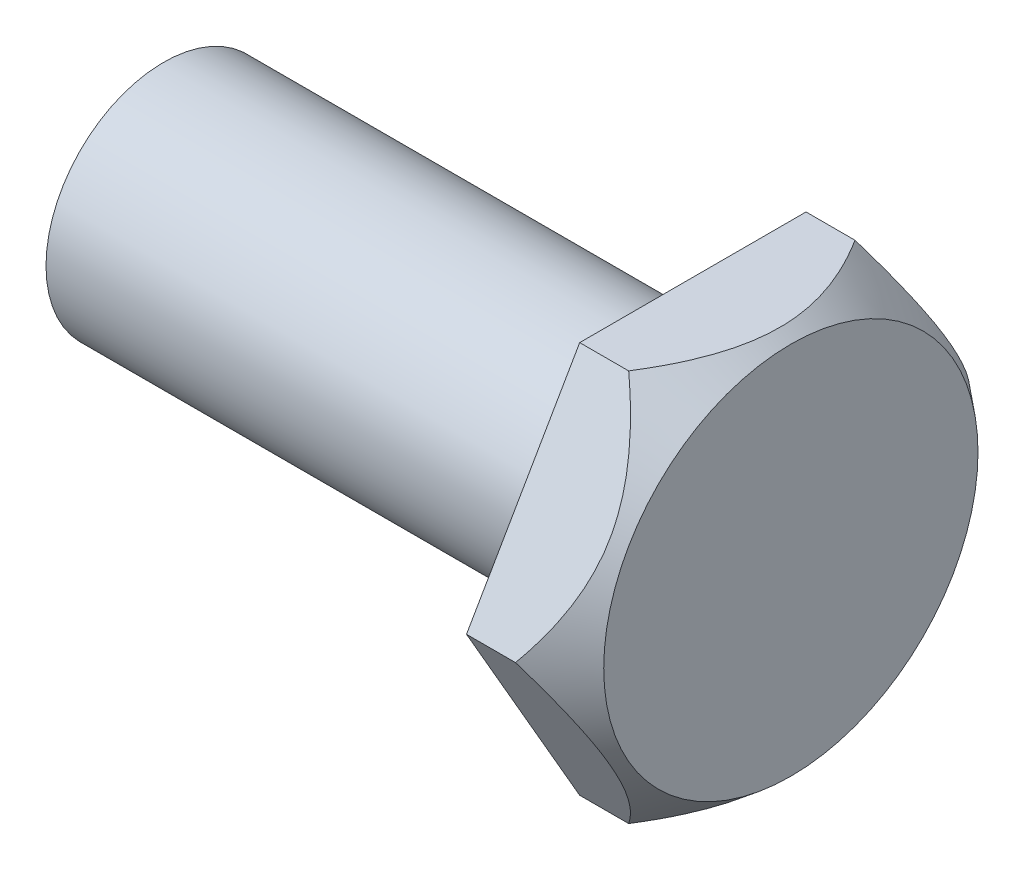
from build123d import *

# Parameters (mm, degrees)
HEX_HEAD_DEPTH     = 5
SHANK_PROFILE_12_R = 6
SHANK_12_DEPTH     = 27


with BuildPart() as part:
    # Hex Head Profile 20AF → Hex Head (new body)
    with BuildSketch(Plane(origin=(0, 0, 0), x_dir=(0, 0, -1), z_dir=(1, 0, 0))):
        Polygon((11.547005384, 0), (5.773502692, 10), (-5.773502692, 10), (-11.547005384, 0), (-5.773502692, -10), (5.773502692, -10), align=None)
    extrude(amount=HEX_HEAD_DEPTH)

    # Shank Profile Ø12 → Shank Ø12 (add)
    with BuildSketch(Plane.ZY):
        Circle(SHANK_PROFILE_12_R)
    extrude(amount=SHANK_12_DEPTH)

    # Head Chamfer Profile → Head Chamfer (revolve, cut)
    with BuildSketch(Plane(origin=(0, 0, 0), x_dir=(1, 0, 0), z_dir=(0, 1, 0)), mode=Mode.PRIVATE) as head_chamfer_sk:
        Polygon((2.5, 11.547005384), (5, 9.547005384), (5, 11.547005384), align=None)
    revolve(head_chamfer_sk.sketch.rotate(Axis((0, 0, 0), (1, 0, 0)), 180), axis=Axis((0, 0, 0), (1, 0, 0)), mode=Mode.SUBTRACT)


solid = part.part
